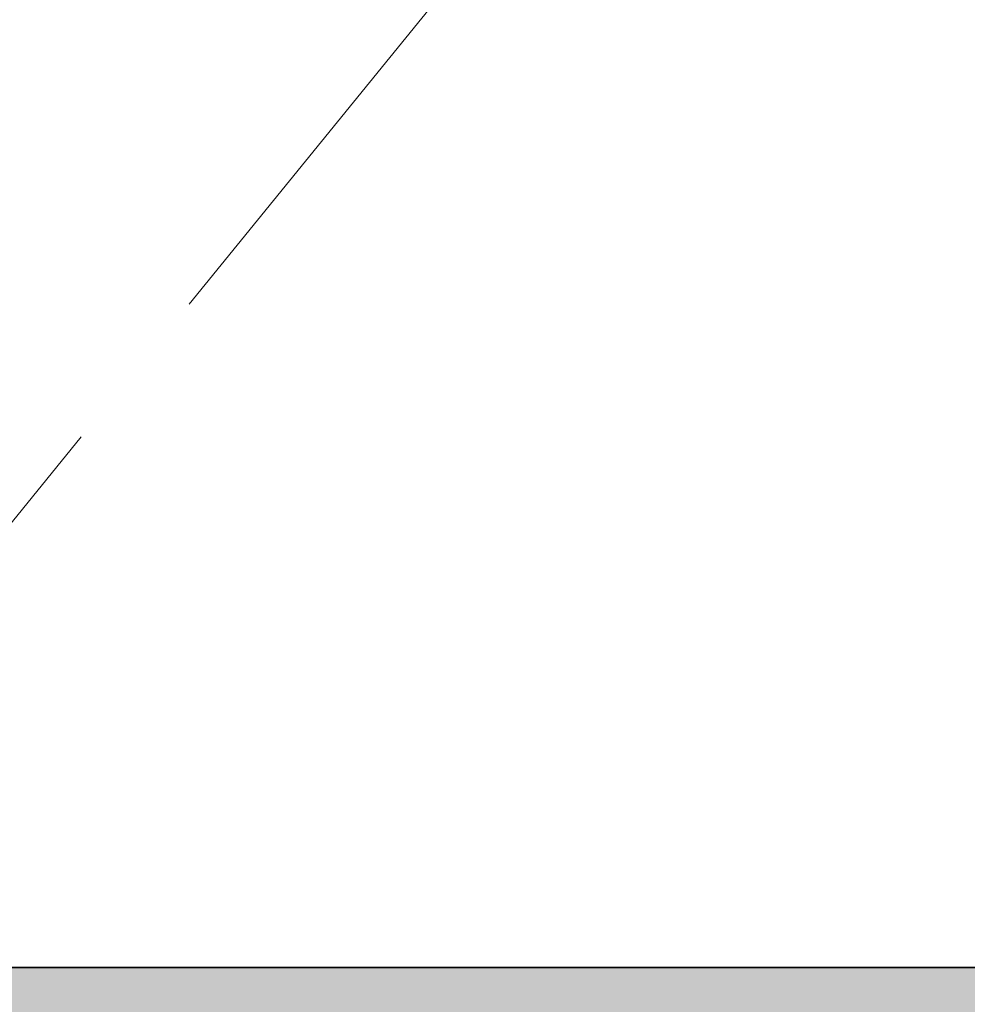
# Model space of a CAD drawing. Units: inches. Extents: x 2083 to 3317, y 1141 to 2115.
# Tile 77 of 256: x 2242.45 to 2259.08, y 1477.12 to 1494.39. Entities that reach past the tile are written whole.
import ezdxf

# ---------------------------------------------------------------- set-up
doc = ezdxf.new("R2010")
doc.units = ezdxf.units.IN
doc.linetypes.add('ACAD_ISO02W100', pattern=[15, 12, -3])
for name, color, linetype, lineweight in [('A-ANNO-DIMS', 2, 'Continuous', 18), ('A-FLOR-OPEN', 8, 'ACAD_ISO02W100', 13), ('A-WALL', 7, 'Continuous', 35)]:
    doc.layers.add(name, color=color, linetype=linetype, lineweight=lineweight)
doc.layers.add('A-WALL-PATT', color=251, linetype='Continuous', lineweight=13, true_color=0x636466)
doc.styles.get("Standard").update_dxf_attribs({"font": 'arial.ttf'})
doc.dimstyles.new('ISO-25', dxfattribs={"dimtxt": 12, "dimasz": 12, "dimexe": 1.25, "dimexo": 0.625, "dimtad": 1, "dimlunit": 3, "dimtxsty": 'Standard', "dimcen": 2.5, "dimadec": 0, "dimazin": 0, "dimtfac": 1, "dimtmove": 0, "dimatfit": 3, "dimfxl": 1, "dimarcsym": 0})

# ---------------------------------------------------------------- blocks, each defined once
blk = doc.blocks.new('*D30')
at = {"layer": 'A-ANNO-DIMS', "color": 0, "lineweight": -2, "transparency": 16777216}
for p, q in [((2240.018, 1445.274), (2240.018, 1448.046)), ((2254.329, 1445.274), (2254.329, 1448.046)), ((2228.018, 1446.796), (2216.018, 1446.796)), ((2240.018, 1446.796), (2254.329, 1446.796)), ((2266.329, 1446.796), (2413.765, 1446.796))]:
    blk.add_line(p, q, dxfattribs=at)
at = {"layer": 'A-ANNO-DIMS', "color": 0, "transparency": 16777216}
for points in [[(2228.018, 1448.796), (2228.018, 1444.796), (2240.018, 1446.796)], [(2266.329, 1448.796), (2266.329, 1444.796), (2254.329, 1446.796)]]:
    blk.add_solid(points, dxfattribs=at)
at = {"layer": 'Defpoints', "color": 0, "transparency": 16777216}
for p in [(2254.329, 1446.796), (2240.018, 1444.649), (2254.329, 1444.649)]:
    blk.add_point(p, dxfattribs=at)
at = {"layer": 'A-ANNO-DIMS', "color": 0, "transparency": 16777216, "insert": (2346.047, 1453.625), "char_height": 12, "attachment_point": 5}
blk.add_mtext('WC 1\'-2 1/2" TYP.', dxfattribs=at)
blk = doc.blocks.new('*D31')
at = {"layer": 'A-ANNO-DIMS', "color": 0, "lineweight": -2, "transparency": 16777216}
for p, q in [((2237.871, 1456.649), (2237.871, 1541.915)), ((2239.393, 1444.649), (2236.621, 1444.649)), ((2237.871, 1431.548), (2237.871, 1444.649)), ((2239.393, 1431.548), (2236.621, 1431.548)), ((2237.871, 1419.548), (2237.871, 1407.548))]:
    blk.add_line(p, q, dxfattribs=at)
at = {"layer": 'A-ANNO-DIMS', "color": 0, "transparency": 16777216}
for points in [[(2235.871, 1456.649), (2239.871, 1456.649), (2237.871, 1444.649)], [(2235.871, 1419.548), (2239.871, 1419.548), (2237.871, 1431.548)]]:
    blk.add_solid(points, dxfattribs=at)
at = {"layer": 'Defpoints', "color": 0, "transparency": 16777216}
for p in [(2237.871, 1444.649), (2240.018, 1444.649), (2240.018, 1431.548)]:
    blk.add_point(p, dxfattribs=at)
at = {"layer": 'A-ANNO-DIMS', "color": 0, "transparency": 16777216, "insert": (2231.217, 1505.282), "char_height": 12, "attachment_point": 5, "rotation": 90}
blk.add_mtext('1\'-1" TYP.', dxfattribs=at)
blk = doc.blocks.new('*D45')
at = {"layer": 'A-ANNO-DIMS', "color": 0, "lineweight": -2, "transparency": 16777216}
for p, q in [((2235.96, 1478.386), (2235.96, 1531.361)), ((2418.96, 1478.386), (2418.96, 1531.361)), ((2247.96, 1530.111), (2406.96, 1530.111))]:
    blk.add_line(p, q, dxfattribs=at)
at = {"layer": 'A-ANNO-DIMS', "color": 0, "transparency": 16777216}
for points in [[(2247.96, 1532.111), (2247.96, 1528.111), (2235.96, 1530.111)], [(2406.96, 1532.111), (2406.96, 1528.111), (2418.96, 1530.111)]]:
    blk.add_solid(points, dxfattribs=at)
at = {"layer": 'Defpoints', "color": 0, "transparency": 16777216}
for p in [(2418.96, 1530.111), (2235.96, 1477.761), (2418.96, 1477.761)]:
    blk.add_point(p, dxfattribs=at)
at = {"layer": 'A-ANNO-DIMS', "color": 0, "transparency": 16777216, "insert": (2327.46, 1536.867), "char_height": 12, "attachment_point": 5}
blk.add_mtext('15\'-3"', dxfattribs=at)
blk = doc.blocks.new('*D62')
at = {"layer": 'A-ANNO-DIMS', "color": 0, "lineweight": -2, "transparency": 16777216}
for p, q in [((2235.96, 1469.386), (2235.96, 1522.361)), ((2379.96, 1469.386), (2379.96, 1522.361)), ((2247.96, 1521.111), (2367.96, 1521.111))]:
    blk.add_line(p, q, dxfattribs=at)
at = {"layer": 'A-ANNO-DIMS', "color": 0, "transparency": 16777216}
for points in [[(2247.96, 1523.111), (2247.96, 1519.111), (2235.96, 1521.111)], [(2367.96, 1523.111), (2367.96, 1519.111), (2379.96, 1521.111)]]:
    blk.add_solid(points, dxfattribs=at)
at = {"layer": 'Defpoints', "color": 0, "transparency": 16777216}
for p in [(2379.96, 1521.111), (2235.96, 1468.761), (2379.96, 1468.761)]:
    blk.add_point(p, dxfattribs=at)
at = {"layer": 'A-ANNO-DIMS', "color": 0, "transparency": 16777216, "insert": (2307.96, 1527.863), "char_height": 12, "attachment_point": 5}
blk.add_mtext('12\'-0"', dxfattribs=at)
blk = doc.blocks.new('*D64')
at = {"layer": 'A-ANNO-DIMS', "color": 0, "lineweight": -2, "transparency": 16777216}
for p, q in [((2236.585, 1702.761), (2289.56, 1702.761)), ((2288.31, 1690.761), (2288.31, 1489.761)), ((2236.585, 1477.761), (2289.56, 1477.761))]:
    blk.add_line(p, q, dxfattribs=at)
at = {"layer": 'A-ANNO-DIMS', "color": 0, "transparency": 16777216}
for points in [[(2286.31, 1690.761), (2290.31, 1690.761), (2288.31, 1702.761)], [(2286.31, 1489.761), (2290.31, 1489.761), (2288.31, 1477.761)]]:
    blk.add_solid(points, dxfattribs=at)
at = {"layer": 'Defpoints', "color": 0, "transparency": 16777216}
for p in [(2235.96, 1702.761), (2235.96, 1477.761), (2288.31, 1477.761)]:
    blk.add_point(p, dxfattribs=at)
at = {"layer": 'A-ANNO-DIMS', "color": 0, "transparency": 16777216, "insert": (2281.558, 1590.261), "char_height": 12, "attachment_point": 5, "rotation": 90}
blk.add_mtext('18\'-9"', dxfattribs=at)

msp = doc.modelspace()

# ---------------------------------------------------------------- hatches: boundary and pattern name
at = {"layer": 'A-WALL-PATT'}
h = msp.add_hatch(color=256, dxfattribs=at)
h.dxf.hatch_style = 1
h.paths.add_polyline_path([(3126.96, 2020.761), (2748.96, 2020.761), (2604.96, 2020.761), (2226.96, 2020.761), (2226.96, 1702.761), (2466.96, 1702.761), (2466.96, 1582.761), (2418.96, 1582.761), (2418.96, 1477.761), (2226.96, 1477.761), (2226.96, 1263.261), (2544.96, 1263.261), (2544.96, 1411.761), (2604.96, 1411.761), (2685.96, 1411.761), (2685.96, 1420.761), (2604.96, 1420.761), (2604.96, 1573.761), (2604.96, 1702.761), (2604.96, 2011.761), (2748.96, 2011.761), (2748.96, 1702.761), (2862.96, 1702.761), (2862.96, 1621.761), (2871.96, 1621.761), (2871.96, 1702.761), (2883.96, 1702.761), (2883.96, 1706.939, -0.026459), (2883.96, 1711.761), (2757.96, 1711.761), (2757.96, 1807.761), (2787.96, 1807.761), (2787.96, 1812.261), (2757.96, 1812.261), (2757.96, 2011.761), (2877.96, 2011.761), (2877.96, 1812.261), (2847.96, 1812.261), (2847.96, 1807.761), (2889.836, 1807.761), (2889.836, 1812.261), (2882.46, 1812.261), (2882.46, 2011.761), (3117.96, 2011.761), (3117.96, 1812.261), (2937.836, 1812.261), (2937.836, 1807.761), (2995.71, 1807.761), (2995.71, 1796.118), (3000.21, 1796.118), (3000.21, 1807.761), (3117.96, 1807.761), (3117.96, 1711.761), (3000.21, 1711.761), (3000.21, 1760.118), (2998.573, 1760.118, -0.020711), (2995.71, 1760.118), (2995.71, 1711.761), (2931.96, 1711.761), (2931.96, 1702.761), (3126.96, 1702.761)])
h.paths.add_polyline_path([(2471.46, 2011.761), (2471.46, 1810.011), (2462.717, 1810.011), (2462.717, 1805.511), (2505.96, 1805.511), (2505.96, 1810.011), (2475.96, 1810.011), (2475.96, 2011.761), (2595.96, 2011.761), (2595.96, 1810.011), (2565.96, 1810.011), (2565.96, 1805.511), (2595.96, 1805.511), (2595.96, 1711.761), (2235.96, 1711.761), (2235.96, 1805.511), (2353.71, 1805.511), (2353.71, 1796.054), (2358.21, 1796.054), (2358.21, 1805.511), (2414.717, 1805.511), (2414.717, 1810.011), (2235.96, 1810.011), (2235.96, 2011.761)], flags=16)
h.paths.add_polyline_path([(2270.205, 1994.61), (2270.205, 1970.61), (2246.205, 1970.61), (2246.205, 1994.61)], flags=0)
edge = h.paths.add_edge_path(flags=0)
edge.add_ellipse((2332.027, 1899.798), major_axis=(-3.043, 3.043), ratio=0.168252, start_angle=-161.3322, end_angle=-156.3071, ccw=False)
edge.add_ellipse((2333.082, 1898.744), major_axis=(-1.055, 1.055), ratio=0.453532, start_angle=-123.371, end_angle=-94.1591)
edge = h.paths.add_edge_path(flags=0)
edge.add_ellipse((2332.027, 1968.876), major_axis=(3.043, 3.043), ratio=0.168252, start_angle=18.6678, end_angle=23.6929)
edge.add_spline(control_points=[(2332.926, 1970.691), (2332.227, 1970.336), (2330.894, 1969.659), (2328.413, 1970.932), (2327.204, 1967.749), (2324.71, 1969.956), (2322.533, 1967.012), (2320.013, 1971.296), (2317.68, 1968.158), (2316.041, 1967.102), (2315.427, 1966.81)], knot_values=[0, 0, 0, 0, 2.267059, 4.324559, 6.685584, 8.878641, 11.121502, 14.300359, 17.755284, 19.732645, 19.732645, 19.732645, 19.732645], degree=3, periodic=0)
edge.add_ellipse((2332.027, 1968.876), major_axis=(3.043, 3.043), ratio=0.168252, start_angle=18.6678, end_angle=23.6929, ccw=False)
edge.add_ellipse((2333.082, 1969.931), major_axis=(1.055, 1.055), ratio=0.453532, start_angle=56.629, end_angle=85.8409, ccw=False)
edge = h.paths.add_edge_path(flags=0)
edge.add_spline(control_points=[(2296.428, 1967.988), (2293.628, 1965.336), (2287.704, 1959.727), (2299.744, 1949.996), (2294.533, 1935.669), (2290.573, 1920.604), (2293.394, 1909.974), (2296.185, 1904.967)], knot_values=[0.099185, 0.099185, 0.099185, 0.099185, 0.345301, 0.619822, 0.982653, 1.386093, 1.810555, 1.810555, 1.810555, 1.810555], degree=3, periodic=0)
edge.add_spline(control_points=[(2296.185, 1904.967), (2297.384, 1902.619), (2298.001, 1901.949), (2298.553, 1901.468)], knot_values=[0.006246, 0.006246, 0.006246, 0.006246, 0.055476, 0.055476, 0.055476, 0.055476], degree=3, periodic=0)
edge.add_spline(control_points=[(2298.553, 1901.468), (2297.259, 1900.923), (2295.225, 1900.232), (2293.06, 1900.614), (2292.101, 1900.788), (2292.09, 1900.791)], knot_values=[0.312835, 0.312835, 0.312835, 0.312835, 0.40178, 0.474987, 0.475903, 0.475903, 0.475903, 0.475903], degree=3, periodic=0)
edge.add_arc((2292.794, 1904.664), 3.937, 215.4209, 259.6982, ccw=False)
edge.add_spline(control_points=[(2289.585, 1902.382), (2289.477, 1902.535), (2289.368, 1902.688), (2289.261, 1902.841)], knot_values=[0.102872, 0.102872, 0.102872, 0.102872, 0.116896, 0.116896, 0.116896, 0.116896], degree=3, periodic=0)
edge.add_spline(control_points=[(2289.261, 1902.841), (2288.687, 1902.55), (2287.64, 1902.02), (2285.881, 1901.874), (2283.853, 1901.504), (2281.72, 1899.711), (2278.467, 1899.493), (2276.157, 1901.883), (2272.259, 1899.804), (2267.778, 1901.843), (2262.244, 1900.184), (2257.415, 1901.782), (2254.318, 1900.726), (2253.178, 1900.337)], knot_values=[0, 0, 0, 0, 1.907977, 3.477176, 5.261074, 7.972851, 11.680248, 13.717921, 16.939592, 22.789562, 27.502503, 33.595215, 37.145618, 37.145618, 37.145618, 37.145618], degree=3, periodic=0)
edge.add_line((2253.178, 1900.337), (2250.244, 1902.841))
edge.add_line((2250.244, 1902.841), (2250.244, 1965.833))
edge.add_line((2250.244, 1965.833), (2253.178, 1968.337))
edge.add_spline(control_points=[(2253.178, 1968.337), (2254.318, 1967.948), (2257.415, 1966.892), (2262.244, 1968.49), (2267.778, 1966.831), (2271.527, 1968.537), (2273.876, 1967.828), (2274.207, 1967.728)], knot_values=[0, 0, 0, 0, 0.09018, 0.244935, 0.364644, 0.513233, 0.537855, 0.537855, 0.537855, 0.537855], degree=3, periodic=0)
edge.add_arc((2274.353, 1963.793), 3.937, 72.0511, 92.1279, ccw=False)
edge.add_arc((2281.297, 1985.23), 18.596, 252.0511, 288.5657)
edge.add_arc((2292.317, 1956.029), 12.646, 71.0268, 113.7782, ccw=False)
edge = h.paths.add_edge_path(flags=0)
edge.add_spline(control_points=[(2274.899, 1951.856), (2275.066, 1951.617), (2275.233, 1951.377), (2275.398, 1951.136)], knot_values=[1.409916, 1.409916, 1.409916, 1.409916, 1.43159, 1.43159, 1.43159, 1.43159], degree=3, periodic=0)
edge.add_spline(control_points=[(2275.398, 1951.136), (2275.792, 1950.562), (2276.179, 1949.984), (2276.546, 1949.397)], knot_values=[1.358238, 1.358238, 1.358238, 1.358238, 1.409916, 1.409916, 1.409916, 1.409916], degree=3, periodic=0)
edge.add_line((2276.546, 1949.397), (2277.437, 1947.862))
edge.add_spline(control_points=[(2277.437, 1947.862), (2276.304, 1945.673), (2274.64, 1942.427), (2274.632, 1938.094), (2272.799, 1930.852), (2274.356, 1943.897), (2275.948, 1947.923), (2276.546, 1949.397)], knot_values=[0.005632, 0.005632, 0.005632, 0.005632, 0.186014, 0.266002, 0.357087, 0.59639, 0.739732, 0.739732, 0.739732, 0.739732], degree=3, periodic=0)
edge.add_spline(control_points=[(2276.546, 1949.397), (2276.179, 1949.984), (2275.792, 1950.562), (2275.398, 1951.136)], knot_values=[1.358238, 1.358238, 1.358238, 1.358238, 1.409916, 1.409916, 1.409916, 1.409916], degree=3, periodic=0)
edge.add_spline(control_points=[(2275.398, 1951.136), (2274.943, 1950.08), (2274.208, 1948.025), (2273.935, 1944.851), (2272.469, 1937.627), (2273.466, 1945.696), (2274.701, 1951.059), (2274.899, 1951.856)], knot_values=[0.104364, 0.104364, 0.104364, 0.104364, 0.189636, 0.269624, 0.36071, 0.600013, 0.644622, 0.644622, 0.644622, 0.644622], degree=3, periodic=0)
h.paths.add_polyline_path([(2269.168, 1963.128, -0.357527), (2268.171, 1960.976, -0.092561), (2268.171, 1939.436, -0.357527), (2269.168, 1937.285, -0.357527), (2267.016, 1938.282, -0.164785), (2254.686, 1938.282, -0.357527), (2252.534, 1937.285, -0.357527), (2253.531, 1939.436, -0.092561), (2253.531, 1960.976, -0.357527), (2252.534, 1963.128, -0.357527), (2254.686, 1962.131, -0.164785), (2267.016, 1962.131, -0.357527)], flags=0)
h.paths.add_polyline_path([(2248.874, 1967.802), (2248.874, 1957.028), (2249.458, 1957.028), (2249.458, 1911.647), (2248.874, 1911.647), (2248.874, 1900.873), (2246.512, 1900.873, 0.197327), (2244.15, 1902.457), (2244.15, 1966.218, 0.197327), (2246.512, 1967.802)], flags=0)
h.paths.add_polyline_path([(2269.168, 1931.389, -0.357527), (2268.171, 1929.238, -0.092561), (2268.171, 1907.698, -0.357527), (2269.168, 1905.547, -0.357527), (2267.016, 1906.544, -0.164785), (2254.686, 1906.544, -0.357527), (2252.534, 1905.547, -0.357527), (2253.531, 1907.698, -0.092561), (2253.531, 1929.238, -0.357527), (2252.534, 1931.389, -0.357527), (2254.686, 1930.392, -0.164785), (2267.016, 1930.392, -0.357527)], flags=0)
edge = h.paths.add_edge_path(flags=0)
edge.add_spline(control_points=[(2276.197, 1906.724), (2276.168, 1909.029), (2276.114, 1913.372), (2270.598, 1924.925), (2273.905, 1919.013), (2275.922, 1916.262), (2275.475, 1912.402), (2277.258, 1910.381), (2276.696, 1908.225), (2276.646, 1906.813), (2276.618, 1906.008)], knot_values=[0, 0, 0, 0, 8.61026, 16.221274, 18.843057, 23.804898, 27.440828, 29.356102, 31.203478, 33.650687, 33.650687, 33.650687, 33.650687], degree=3, periodic=0)
edge.add_spline(control_points=[(2276.618, 1906.008), (2276.623, 1905.624), (2276.498, 1904.629), (2275.442, 1903.855), (2274.937, 1903.08), (2274.859, 1902.841)], knot_values=[0.156488, 0.156488, 0.156488, 0.156488, 0.184398, 0.231376, 0.250598, 0.250598, 0.250598, 0.250598], degree=3, periodic=0)
edge.add_line((2274.859, 1902.841), (2276.506, 1902.841))
edge.add_spline(control_points=[(2276.506, 1902.841), (2276.788, 1903.085), (2277.665, 1904.125), (2278.25, 1904.341), (2277.654, 1908.527), (2278.156, 1906.228), (2278.1, 1905.286), (2278.847, 1904.069), (2277.857, 1903.415), (2277.874, 1902.991), (2277.904, 1902.841)], knot_values=[0.059574, 0.059574, 0.059574, 0.059574, 0.080753, 0.103741, 0.16972, 0.176036, 0.207137, 0.240474, 0.262341, 0.27366, 0.27366, 0.27366, 0.27366], degree=3, periodic=0)
edge.add_line((2277.904, 1902.841), (2280.03, 1902.841))
edge.add_spline(control_points=[(2280.03, 1902.841), (2279.888, 1903.088), (2279.499, 1903.982), (2280.152, 1905.939), (2278.104, 1909.658), (2279.762, 1907.185), (2280.328, 1904.875), (2280.485, 1903.49), (2281.463, 1903.249), (2281.758, 1902.936), (2281.834, 1902.841)], knot_values=[0.013856, 0.013856, 0.013856, 0.013856, 0.034874, 0.088867, 0.107879, 0.126738, 0.158714, 0.193757, 0.217487, 0.226722, 0.226722, 0.226722, 0.226722], degree=3, periodic=0)
edge.add_spline(control_points=[(2281.834, 1902.841), (2281.788, 1902.827), (2281.647, 1902.783), (2281.396, 1902.859), (2281.088, 1902.985), (2280.721, 1903.061), (2280.333, 1903.026), (2280.125, 1902.899), (2280.03, 1902.841)], knot_values=[0, 0, 0, 0, 0.14413, 0.435517, 0.749276, 1.153046, 1.548371, 1.878348, 1.878348, 1.878348, 1.878348], degree=3, periodic=0)
edge.add_line((2280.03, 1902.841), (2277.904, 1902.841))
edge.add_spline(control_points=[(2277.904, 1902.841), (2277.893, 1902.796), (2277.865, 1902.68), (2277.607, 1902.687), (2277.274, 1902.801), (2276.838, 1902.62), (2276.584, 1902.789), (2276.506, 1902.841)], knot_values=[0, 0, 0, 0, 0.127189, 0.326199, 0.628009, 1.24357, 1.515331, 1.515331, 1.515331, 1.515331], degree=3, periodic=0)
edge.add_line((2276.506, 1902.841), (2274.859, 1902.841))
edge.add_spline(control_points=[(2274.859, 1902.841), (2274.814, 1902.899), (2274.725, 1903.013), (2274.493, 1903.119), (2274.244, 1902.961), (2273.937, 1903.185), (2273.614, 1902.983), (2273.408, 1902.883), (2273.322, 1902.841)], knot_values=[0, 0, 0, 0, 0.21843, 0.436957, 0.687977, 0.990379, 1.398396, 1.69185, 1.69185, 1.69185, 1.69185], degree=3, periodic=0)
edge.add_spline(control_points=[(2273.322, 1902.841), (2273.617, 1903.446), (2274.274, 1904.538), (2276.027, 1904.574), (2276.207, 1906.584), (2276.197, 1906.724)], knot_values=[0.012227, 0.012227, 0.012227, 0.012227, 0.059472, 0.106218, 0.134458, 0.134458, 0.134458, 0.134458], degree=3, periodic=0)
h.paths.add_polyline_path([(2270.776, 1897.79), (2270.776, 1873.79), (2246.776, 1873.79), (2246.776, 1897.79)], flags=0)
h.paths.add_polyline_path([(2353.71, 1760.005), (2353.71, 1760.054), (2358.21, 1760.054, -0.033729)], flags=0)
h.paths.add_polyline_path([(2321.819, 1737.529), (2341.995, 1737.529, -0.414214), (2343.203, 1736.321), (2343.203, 1721.021, -0.414214), (2341.995, 1719.813), (2321.819, 1719.813, -0.414214), (2320.611, 1721.021), (2320.611, 1736.321, -0.414214)], flags=0)
h.paths.add_polyline_path([(2324.235, 1736.321), (2339.579, 1736.321, -0.414214), (2341.995, 1733.905), (2341.995, 1725.45, -0.414214), (2339.579, 1723.034), (2333.681, 1723.034), (2333.845, 1722.045, -0.870646), (2335.425, 1721.826, -0.767327), (2333.923, 1721.423), (2331.291, 1721.423, -0.767327), (2329.788, 1721.826, -0.870646), (2331.368, 1722.045), (2331.533, 1723.034), (2324.235, 1723.034, -0.414214), (2321.819, 1725.45), (2321.819, 1733.905, -0.414214)], flags=0)
h.paths.add_polyline_path([(2570.484, 1928.615), (2589.684, 1928.615), (2590.169, 1928.615), (2590.169, 1904.993), (2570.484, 1904.993)], flags=0)
h.paths.add_polyline_path([(2574.447, 1927.264, -1), (2572.829, 1927.264, -1)], flags=0)
h.paths.add_polyline_path([(2573.09, 1926.941), (2573.925, 1927.776), (2574.148, 1927.553), (2573.313, 1926.718)], flags=0)
h.paths.add_polyline_path([(2578.779, 1919.73, -1), (2571.592, 1919.73, -1)], flags=0)
h.paths.add_polyline_path([(2578.385, 1919.73, -1), (2571.985, 1919.73, -1)], flags=0)
h.paths.add_polyline_path([(2331.596, 1729.476, -1), (2333.618, 1729.476, -1)], flags=0)
h.paths.add_polyline_path([(2578.034, 1927.264, -1), (2576.416, 1927.264, -1)], flags=0)
h.paths.add_polyline_path([(2576.689, 1927.531), (2576.912, 1927.754), (2577.747, 1926.919), (2577.524, 1926.696)], flags=0)
h.paths.add_polyline_path([(2578.139, 1909.86, -1), (2572.232, 1909.86, -1)], flags=0)
h.paths.add_polyline_path([(2577.745, 1909.86, -1), (2572.625, 1909.86, -1)], flags=0)
h.paths.add_polyline_path([(2583.798, 1927.264, -1), (2582.179, 1927.264, -1)], flags=0)
h.paths.add_polyline_path([(2582.719, 1927.754), (2583.554, 1926.919), (2583.331, 1926.696), (2582.496, 1927.531)], flags=0)
h.paths.add_polyline_path([(2582.496, 1927.531), (2582.719, 1927.754), (2583.554, 1926.919), (2583.331, 1926.696)], flags=0)
h.paths.add_polyline_path([(2587.739, 1920.53, -1), (2581.832, 1920.53, -1)], flags=0)
h.paths.add_polyline_path([(2587.345, 1920.53, -1), (2582.225, 1920.53, -1)], flags=0)
h.paths.add_polyline_path([(2587.385, 1927.264, -1), (2585.766, 1927.264, -1)], flags=0)
h.paths.add_polyline_path([(2586.082, 1926.98), (2586.917, 1927.815), (2587.14, 1927.593), (2586.305, 1926.758)], flags=0)
h.paths.add_polyline_path([(2588.379, 1910.66, -1), (2581.192, 1910.66, -1)], flags=0)
h.paths.add_polyline_path([(2587.985, 1910.66, -1), (2581.585, 1910.66, -1)], flags=0)
h.paths.add_polyline_path([(2417.168, 1729.478), (2437.344, 1729.478, -0.414214), (2438.552, 1728.27), (2438.552, 1712.969, -0.414214), (2437.344, 1711.761), (2417.168, 1711.761, -0.414214), (2415.96, 1712.969), (2415.96, 1728.27, -0.414214)], flags=0)
h.paths.add_polyline_path([(2419.584, 1728.27), (2434.928, 1728.27, -0.414214), (2437.344, 1725.854), (2437.344, 1717.398, -0.414214), (2434.928, 1714.983), (2429.029, 1714.983), (2429.194, 1713.994, -0.870646), (2430.774, 1713.775, -0.767327), (2429.271, 1713.372), (2426.64, 1713.372, -0.767327), (2425.137, 1713.775, -0.870646), (2426.717, 1713.994), (2426.882, 1714.983), (2419.584, 1714.983, -0.414214), (2417.168, 1717.398), (2417.168, 1725.854, -0.414214)], flags=0)
h.paths.add_polyline_path([(2419.584, 1728.27), (2434.928, 1728.27, -0.414214), (2437.344, 1725.854), (2437.344, 1717.398, -0.414214), (2434.928, 1714.983), (2429.029, 1714.983), (2428.358, 1719.009), (2427.553, 1719.009), (2426.882, 1714.983), (2419.584, 1714.983, -0.414214), (2417.168, 1717.398), (2417.168, 1725.854, -0.414214)], flags=0)
h.paths.add_polyline_path([(2426.944, 1721.425, -1), (2428.967, 1721.425, -1)], flags=0)
h.paths.add_polyline_path([(2475.96, 1702.761), (2595.96, 1702.761), (2595.96, 1582.761), (2475.96, 1582.761)], flags=16)
h.paths.add_polyline_path([(2427.96, 1573.761), (2595.96, 1573.761), (2595.96, 1468.761), (2595.96, 1420.761), (2384.46, 1420.761), (2384.46, 1468.761), (2427.96, 1468.761)], flags=16)
h.paths.add_polyline_path([(2379.96, 1468.761), (2379.96, 1420.761), (2235.96, 1420.761), (2235.96, 1468.761)], flags=16)
h.paths.add_polyline_path([(2317.816, 1466.696), (2337.992, 1466.696, -0.414214), (2339.2, 1465.488), (2339.2, 1450.187, -0.414214), (2337.992, 1448.979), (2317.816, 1448.979, -0.414214), (2316.608, 1450.187), (2316.608, 1465.488, -0.414214)], flags=0)
h.paths.add_polyline_path([(2320.232, 1465.488), (2335.576, 1465.488, -0.414214), (2337.992, 1463.072), (2337.992, 1454.616, -0.414214), (2335.576, 1452.2), (2329.677, 1452.2), (2329.842, 1451.212, -0.870646), (2331.422, 1450.992, -0.767327), (2329.92, 1450.59), (2327.288, 1450.59, -0.767327), (2325.785, 1450.992, -0.870646), (2327.365, 1451.212), (2327.53, 1452.2), (2320.232, 1452.2, -0.414214), (2317.816, 1454.616), (2317.816, 1463.072, -0.414214)], flags=0)
h.paths.add_polyline_path([(2320.232, 1465.488), (2335.576, 1465.488, -0.414214), (2337.992, 1463.072), (2337.992, 1454.616, -0.414214), (2335.576, 1452.2), (2329.677, 1452.2), (2329.006, 1456.227), (2328.201, 1456.227), (2327.53, 1452.2), (2320.232, 1452.2, -0.414214), (2317.816, 1454.616), (2317.816, 1463.072, -0.414214)], flags=0)
h.paths.add_polyline_path([(2327.593, 1458.643, -1), (2329.615, 1458.643, -1)], flags=0)
h.paths.add_polyline_path([(2244.412, 1433.34), (2241.921, 1433.34, -0.414214), (2240.018, 1435.244), (2240.018, 1440.953, -0.414211), (2241.921, 1442.856), (2244.412, 1442.856, -1.976472)], flags=0)
h.paths.add_polyline_path([(2245.357, 1434.398, -0.414214), (2245.357, 1441.799, -2.144098)], flags=0)
h.paths.add_polyline_path([(2535.96, 1416.261), (2535.96, 1272.261), (2235.96, 1272.261), (2235.96, 1416.261)], flags=16)
h.paths.add_polyline_path([(2260.12, 1384.293), (2260.12, 1362.039), (2237.865, 1362.039), (2237.865, 1384.293)], flags=0)
edge = h.paths.add_edge_path(flags=0)
edge.add_line((2318.252, 1362.093), (2318.146, 1362.001))
edge.add_ellipse((2317.445, 1360.431), major_axis=(2.822, 2.822), ratio=0.168252, start_angle=18.6678, end_angle=20.9481, ccw=False)
edge.add_ellipse((2318.423, 1361.409), major_axis=(0.978, 0.978), ratio=0.453532, start_angle=56.629, end_angle=70.2262, ccw=False)
edge = h.paths.add_edge_path(flags=0)
edge.add_line((2319.107, 1295.571), (2319.015, 1295.677))
edge.add_ellipse((2317.445, 1296.378), major_axis=(-2.822, 2.822), ratio=0.168252, start_angle=-161.3322, end_angle=-159.0519, ccw=False)
edge.add_ellipse((2318.423, 1295.4), major_axis=(-0.978, 0.978), ratio=0.453532, start_angle=-123.371, end_angle=-109.7738)
edge = h.paths.add_edge_path(flags=0)
edge.add_spline(control_points=[(2284.21, 1301.17), (2284.581, 1300.445), (2284.891, 1299.892), (2285.16, 1299.461)], knot_values=[0.039066, 0.039066, 0.039066, 0.039066, 0.055476, 0.055476, 0.055476, 0.055476], degree=3, periodic=0)
edge.add_line((2285.16, 1299.461), (2284.21, 1301.17))
edge = h.paths.add_edge_path(flags=0)
edge.add_line((2280.412, 1297.298), (2283.37, 1297.036))
edge.add_line((2283.37, 1297.036), (2286.406, 1297.926))
edge.add_spline(control_points=[(2286.406, 1297.926), (2285.305, 1297.463), (2284.345, 1297.129), (2283.37, 1297.036)], knot_values=[0.394369, 0.394369, 0.394369, 0.394369, 0.475903, 0.475903, 0.475903, 0.475903], degree=3, periodic=0)
edge.add_spline(control_points=[(2283.37, 1297.036), (2283.281, 1297.028), (2282.316, 1296.957), (2281.313, 1297.134), (2280.423, 1297.296), (2280.412, 1297.298)], knot_values=[0.312835, 0.312835, 0.312835, 0.312835, 0.320246, 0.393453, 0.394369, 0.394369, 0.394369, 0.394369], degree=3, periodic=0)
edge = h.paths.add_edge_path(flags=0)
edge.add_line((2284.436, 1359.607), (2280.446, 1355.328))
edge.add_line((2280.446, 1355.328), (2279.58, 1351.018))
edge.add_line((2279.58, 1351.018), (2282.413, 1346.58))
edge.add_spline(control_points=[(2282.413, 1346.58), (2283.153, 1345.589), (2284.253, 1344.029), (2284.801, 1342.387), (2284.935, 1341.806)], knot_values=[1.240098, 1.240098, 1.240098, 1.240098, 1.332892, 1.382712, 1.382712, 1.382712, 1.382712], degree=3, periodic=0)
edge.add_spline(control_points=[(2284.935, 1341.806), (2285.319, 1340.141), (2285.233, 1338.409), (2284.91, 1336.654)], knot_values=[1.097484, 1.097484, 1.097484, 1.097484, 1.240098, 1.240098, 1.240098, 1.240098], degree=3, periodic=0)
edge.add_spline(control_points=[(2284.91, 1336.654), (2284.587, 1334.899), (2284.027, 1333.12), (2283.463, 1331.361)], knot_values=[0.95487, 0.95487, 0.95487, 0.95487, 1.097484, 1.097484, 1.097484, 1.097484], degree=3, periodic=0)
edge.add_line((2283.463, 1331.361), (2281.89, 1326.153))
edge.add_line((2281.89, 1326.153), (2280.756, 1321.056))
edge.add_line((2280.756, 1321.056), (2280.299, 1316.002))
edge.add_line((2280.299, 1316.002), (2280.716, 1310.95))
edge.add_line((2280.716, 1310.95), (2282.028, 1305.972))
edge.add_line((2282.028, 1305.972), (2284.21, 1301.17))
edge.add_spline(control_points=[(2284.21, 1301.17), (2283.341, 1302.73), (2282.612, 1304.336), (2282.028, 1305.972)], knot_values=[0.099185, 0.099185, 0.099185, 0.099185, 0.241799, 0.241799, 0.241799, 0.241799], degree=3, periodic=0)
edge.add_spline(control_points=[(2282.028, 1305.972), (2281.444, 1307.608), (2281.005, 1309.273), (2280.716, 1310.95)], knot_values=[0.241799, 0.241799, 0.241799, 0.241799, 0.384413, 0.384413, 0.384413, 0.384413], degree=3, periodic=0)
edge.add_spline(control_points=[(2280.716, 1310.95), (2280.433, 1312.588), (2280.289, 1314.277), (2280.299, 1315.962), (2280.299, 1316.002)], knot_values=[0.384413, 0.384413, 0.384413, 0.384413, 0.523647, 0.527028, 0.527028, 0.527028, 0.527028], degree=3, periodic=0)
edge.add_spline(control_points=[(2280.299, 1316.002), (2280.312, 1317.687), (2280.478, 1319.368), (2280.756, 1321.056)], knot_values=[0.527028, 0.527028, 0.527028, 0.527028, 0.669642, 0.669642, 0.669642, 0.669642], degree=3, periodic=0)
edge.add_spline(control_points=[(2280.756, 1321.056), (2281.035, 1322.744), (2281.426, 1324.44), (2281.89, 1326.153)], knot_values=[0.669642, 0.669642, 0.669642, 0.669642, 0.812256, 0.812256, 0.812256, 0.812256], degree=3, periodic=0)
edge.add_spline(control_points=[(2281.89, 1326.153), (2282.264, 1327.533), (2282.788, 1329.262), (2283.353, 1331.018), (2283.463, 1331.361)], knot_values=[0.812256, 0.812256, 0.812256, 0.812256, 0.927087, 0.95487, 0.95487, 0.95487, 0.95487], degree=3, periodic=0)
edge.add_line((2283.463, 1331.361), (2284.91, 1336.654))
edge.add_line((2284.91, 1336.654), (2284.935, 1341.806))
edge.add_line((2284.935, 1341.806), (2282.413, 1346.58))
edge.add_spline(control_points=[(2282.413, 1346.58), (2281.275, 1348.104), (2280.078, 1349.57), (2279.58, 1351.018)], knot_values=[1.382712, 1.382712, 1.382712, 1.382712, 1.525326, 1.525326, 1.525326, 1.525326], degree=3, periodic=0)
edge.add_spline(control_points=[(2279.58, 1351.018), (2279.443, 1351.415), (2279.136, 1352.857), (2279.735, 1354.29), (2280.446, 1355.328)], knot_values=[1.525326, 1.525326, 1.525326, 1.525326, 1.564439, 1.667941, 1.667941, 1.667941, 1.667941], degree=3, periodic=0)
edge.add_spline(control_points=[(2280.446, 1355.328), (2281.426, 1356.758), (2282.931, 1358.183), (2284.436, 1359.607)], knot_values=[1.667941, 1.667941, 1.667941, 1.667941, 1.810555, 1.810555, 1.810555, 1.810555], degree=3, periodic=0)
edge.add_arc((2280.623, 1348.518), 11.726, 71.0268, 113.7782)
edge.add_arc((2270.405, 1375.595), 17.244, 252.0511, 288.5657, ccw=False)
edge.add_arc((2263.966, 1355.718), 3.651, 72.0511, 92.1279)
edge.add_arc((2263.966, 1355.718), 3.651, 92.1279, 177.9851)
edge.add_spline(control_points=[(2260.318, 1355.846), (2260.26, 1354.221), (2260.551, 1350.187), (2262.999, 1346.766), (2264.473, 1344.649)], knot_values=[1.43159, 1.43159, 1.43159, 1.43159, 1.564144, 1.770695, 1.770695, 1.770695, 1.770695], degree=3, periodic=0)
edge.add_line((2264.473, 1344.649), (2264.936, 1343.983))
edge.add_spline(control_points=[(2263.801, 1340.248), (2263.843, 1340.514), (2264.067, 1341.756), (2264.513, 1343.002), (2264.935, 1343.981)], knot_values=[0.53657, 0.53657, 0.53657, 0.53657, 0.559349, 0.644622, 0.644622, 0.644622, 0.644622], degree=3, periodic=0)
edge.add_spline(control_points=[(2264.935, 1343.981), (2265.118, 1343.715), (2265.299, 1343.448), (2265.477, 1343.179)], knot_values=[1.384077, 1.384077, 1.384077, 1.384077, 1.409916, 1.409916, 1.409916, 1.409916], degree=3, periodic=0)
edge.add_spline(control_points=[(2265.477, 1343.179), (2265.655, 1342.911), (2265.829, 1342.641), (2265.999, 1342.369)], knot_values=[1.358238, 1.358238, 1.358238, 1.358238, 1.384077, 1.384077, 1.384077, 1.384077], degree=3, periodic=0)
edge.add_line((2265.999, 1342.369), (2266.826, 1340.946))
edge.add_spline(control_points=[(2266.826, 1340.946), (2268.894, 1337.09), (2271.398, 1325.843), (2270.516, 1310.569), (2275.919, 1301.861), (2277.79, 1299.199)], knot_values=[0.116896, 0.116896, 0.116896, 0.116896, 0.472987, 1.050969, 1.313793, 1.313793, 1.313793, 1.313793], degree=3, periodic=0)
edge.add_spline(control_points=[(2277.79, 1299.199), (2277.839, 1299.128), (2277.889, 1299.057), (2277.94, 1298.987)], knot_values=[0.109884, 0.109884, 0.109884, 0.109884, 0.116896, 0.116896, 0.116896, 0.116896], degree=3, periodic=0)
edge.add_line((2277.94, 1298.987), (2277.789, 1299.199))
edge.add_spline(control_points=[(2277.789, 1299.199), (2277.257, 1298.929), (2276.286, 1298.438), (2275.039, 1298.334), (2274.383, 1298.239), (2274.215, 1298.209)], knot_values=[33.12187, 33.12187, 33.12187, 33.12187, 35.029056, 36.598255, 37.144827, 37.144827, 37.144827, 37.144827], degree=3, periodic=0)
edge.add_line((2274.215, 1298.209), (2273.073, 1297.893))
edge.add_spline(control_points=[(2273.073, 1297.893), (2272.323, 1297.58), (2271.039, 1296.511), (2269.248, 1296.226), (2268.423, 1296.375)], knot_values=[26.532584, 26.532584, 26.532584, 26.532584, 29.198919, 31.839101, 31.839101, 31.839101, 31.839101], degree=3, periodic=0)
edge.add_line((2268.423, 1296.375), (2263.879, 1297.458))
edge.add_spline(control_points=[(2263.879, 1297.458), (2263.556, 1297.359), (2261.86, 1296.839), (2260.239, 1297.282), (2258.933, 1297.516)], knot_values=[15.919551, 15.919551, 15.919551, 15.919551, 16.939592, 21.226067, 21.226067, 21.226067, 21.226067], degree=3, periodic=0)
edge.add_line((2258.933, 1297.516), (2254.055, 1297.329))
edge.add_spline(control_points=[(2254.055, 1297.329), (2253.756, 1297.296), (2252.114, 1297.165), (2250.462, 1297.544), (2249.13, 1297.668)], knot_values=[5.306517, 5.306517, 5.306517, 5.306517, 6.276435, 10.613034, 10.613034, 10.613034, 10.613034], degree=3, periodic=0)
edge.add_line((2249.13, 1297.668), (2244.332, 1296.878))
edge.add_line((2244.332, 1296.878), (2241.611, 1299.199))
edge.add_line((2241.611, 1299.199), (2241.611, 1357.609))
edge.add_line((2241.611, 1357.609), (2244.332, 1359.931))
edge.add_line((2244.332, 1359.931), (2252.729, 1359.543))
edge.add_spline(control_points=[(2252.729, 1359.543), (2252.871, 1359.546), (2253.306, 1359.548), (2253.74, 1359.514), (2254.032, 1359.482)], knot_values=[0.233291, 0.233291, 0.233291, 0.233291, 0.244935, 0.268927, 0.268927, 0.268927, 0.268927], degree=3, periodic=0)
edge.add_line((2254.032, 1359.482), (2259.587, 1359.416))
edge.add_spline(control_points=[(2259.587, 1359.416), (2260.677, 1359.629), (2262.073, 1359.897), (2263.524, 1359.459), (2263.83, 1359.366)], knot_values=[0.422516, 0.422516, 0.422516, 0.422516, 0.513233, 0.537855, 0.537855, 0.537855, 0.537855], degree=3, periodic=0)
edge.add_arc((2263.966, 1355.718), 3.651, 72.0511, 92.1279, ccw=False)
edge.add_arc((2270.405, 1375.595), 17.244, 252.0511, 288.5657)
edge.add_arc((2280.623, 1348.518), 11.726, 71.0268, 113.7782, ccw=False)
h.paths.add_polyline_path([(2240.341, 1359.435), (2240.341, 1349.444), (2240.882, 1349.444), (2240.882, 1307.365), (2240.341, 1307.365), (2240.341, 1297.374), (2238.15, 1297.374, 0.197327), (2235.96, 1298.843), (2235.96, 1357.966, 0.197327), (2238.15, 1359.435)], flags=0)
h.paths.add_polyline_path([(2259.158, 1355.101, -0.357527), (2258.233, 1353.106, -0.092561), (2258.233, 1333.133, -0.357527), (2259.158, 1331.138, -0.357527), (2257.163, 1332.062, -0.164785), (2245.729, 1332.062, -0.357527), (2243.735, 1331.138, -0.357527), (2244.659, 1333.133, -0.092561), (2244.659, 1353.106, -0.357527), (2243.735, 1355.101, -0.357527), (2245.729, 1354.176, -0.164785), (2257.163, 1354.176, -0.357527)], flags=0)
edge = h.paths.add_edge_path(flags=0)
edge.add_line((2265.999, 1342.369), (2266.826, 1340.946))
edge.add_line((2266.826, 1340.946), (2265.308, 1337.814))
edge.add_line((2265.308, 1337.814), (2264.358, 1334.653))
edge.add_line((2264.358, 1334.653), (2264.262, 1333.8))
edge.add_spline(control_points=[(2264.262, 1333.8), (2264.208, 1333.187), (2264.162, 1332.366), (2264.007, 1331.414), (2263.969, 1331.202)], knot_values=[0.464444, 0.464444, 0.464444, 0.464444, 0.516691, 0.531608, 0.531608, 0.531608, 0.531608], degree=3, periodic=0)
edge.add_spline(control_points=[(2263.969, 1331.202), (2263.775, 1330.119), (2263.424, 1328.791), (2263.257, 1328.531), (2263.234, 1328.515)], knot_values=[0.372682, 0.372682, 0.372682, 0.372682, 0.44885, 0.464444, 0.464444, 0.464444, 0.464444], degree=3, periodic=0)
edge.add_spline(control_points=[(2263.234, 1328.515), (2263.096, 1328.42), (2263.131, 1329.301), (2263.275, 1330.616)], knot_values=[0.280919, 0.280919, 0.280919, 0.280919, 0.372682, 0.372682, 0.372682, 0.372682], degree=3, periodic=0)
edge.add_spline(control_points=[(2263.275, 1330.616), (2263.419, 1331.93), (2263.672, 1333.677), (2263.97, 1335.315)], knot_values=[0.189157, 0.189157, 0.189157, 0.189157, 0.280919, 0.280919, 0.280919, 0.280919], degree=3, periodic=0)
edge.add_spline(control_points=[(2263.97, 1335.315), (2264.1, 1336.032), (2264.419, 1337.622), (2264.755, 1338.864), (2264.947, 1339.491)], knot_values=[0.097394, 0.097394, 0.097394, 0.097394, 0.137578, 0.189157, 0.189157, 0.189157, 0.189157], degree=3, periodic=0)
edge.add_spline(control_points=[(2264.947, 1339.491), (2265.29, 1340.606), (2265.644, 1341.494), (2265.999, 1342.369)], knot_values=[0.005632, 0.005632, 0.005632, 0.005632, 0.097394, 0.097394, 0.097394, 0.097394], degree=3, periodic=0)
h.paths.add_polyline_path([(2259.158, 1325.671, -0.357527), (2258.233, 1323.676, -0.092561), (2258.233, 1303.703, -0.357527), (2259.158, 1301.708, -0.357527), (2257.163, 1302.633, -0.164785), (2245.729, 1302.633, -0.357527), (2243.735, 1301.708, -0.357527), (2244.659, 1303.703, -0.092561), (2244.659, 1323.676, -0.357527), (2243.735, 1325.671, -0.357527), (2245.729, 1324.747, -0.164785), (2257.163, 1324.747, -0.357527)], flags=0)
edge = h.paths.add_edge_path(flags=0)
edge.add_spline(control_points=[(2261.709, 1317.311), (2261.679, 1317.418), (2261.762, 1317.389), (2262.491, 1316.09), (2262.962, 1315.301)], knot_values=[14.955861, 14.955861, 14.955861, 14.955861, 16.221274, 18.694826, 18.694826, 18.694826, 18.694826], degree=3, periodic=0)
edge.add_spline(control_points=[(2262.962, 1315.301), (2262.99, 1315.254), (2263.702, 1314.067), (2264.349, 1313.127), (2264.73, 1312.164)], knot_values=[18.694826, 18.694826, 18.694826, 18.694826, 18.843057, 22.433791, 22.433791, 22.433791, 22.433791], degree=3, periodic=0)
edge.add_spline(control_points=[(2264.73, 1312.164), (2264.876, 1311.796), (2265.177, 1310.77), (2265.143, 1309.559), (2265.248, 1308.824)], knot_values=[22.433791, 22.433791, 22.433791, 22.433791, 23.804898, 26.172756, 26.172756, 26.172756, 26.172756], degree=3, periodic=0)
edge.add_line((2265.248, 1308.824), (2265.851, 1307.172))
edge.add_spline(control_points=[(2265.851, 1307.172), (2266.065, 1306.822), (2266.384, 1306.332), (2266.424, 1305.781), (2266.42, 1305.611)], knot_values=[28.062562, 28.062562, 28.062562, 28.062562, 29.356102, 29.911721, 29.911721, 29.911721, 29.911721], degree=3, periodic=0)
edge.add_spline(control_points=[(2266.42, 1305.611), (2266.416, 1305.433), (2266.394, 1305.25), (2266.365, 1305.066)], knot_values=[29.911721, 29.911721, 29.911721, 29.911721, 30.497837, 30.497837, 30.497837, 30.497837], degree=3, periodic=0)
edge.add_line((2266.365, 1305.066), (2266.066, 1302.136))
edge.add_spline(control_points=[(2266.066, 1302.136), (2266.071, 1301.78), (2265.998, 1301.2), (2265.663, 1300.759), (2265.509, 1300.586)], knot_values=[0.156488, 0.156488, 0.156488, 0.156488, 0.184398, 0.203543, 0.203543, 0.203543, 0.203543], degree=3, periodic=0)
edge.add_line((2265.509, 1300.586), (2264.435, 1299.199))
edge.add_line((2264.435, 1299.199), (2265.962, 1299.199))
edge.add_line((2265.962, 1299.199), (2267.336, 1301.175))
edge.add_line((2267.336, 1301.175), (2267.312, 1301.986))
edge.add_spline(control_points=[(2267.312, 1301.986), (2267.261, 1302.862), (2267.16, 1303.737), (2267.271, 1303.326)], knot_values=[0.126229, 0.126229, 0.126229, 0.126229, 0.166617, 0.166617, 0.166617, 0.166617], degree=3, periodic=0)
edge.add_spline(control_points=[(2267.271, 1303.326), (2267.28, 1303.294), (2267.31, 1303.175), (2267.373, 1302.884), (2267.406, 1302.683), (2267.418, 1302.601)], knot_values=[0.166617, 0.166617, 0.166617, 0.166617, 0.16972, 0.176036, 0.180765, 0.180765, 0.180765, 0.180765], degree=3, periodic=0)
edge.add_spline(control_points=[(2267.744, 1300.988), (2267.688, 1301.151), (2267.481, 1301.657), (2267.484, 1302.145), (2267.418, 1302.601)], knot_values=[0.180765, 0.180765, 0.180765, 0.180765, 0.193767, 0.220139, 0.220139, 0.220139, 0.220139], degree=3, periodic=0)
edge.add_line((2267.418, 1302.601), (2267.744, 1300.988))
edge.add_spline(control_points=[(2267.744, 1300.988), (2267.832, 1300.732), (2267.932, 1300.31), (2267.555, 1299.975), (2267.429, 1299.829)], knot_values=[0.220139, 0.220139, 0.220139, 0.220139, 0.240474, 0.25489, 0.25489, 0.25489, 0.25489], degree=3, periodic=0)
edge.add_line((2267.429, 1299.829), (2267.258, 1299.199))
edge.add_line((2267.258, 1299.199), (2269.23, 1299.199))
edge.add_spline(control_points=[(2269.23, 1299.199), (2269.099, 1299.429), (2268.843, 1300.016), (2269.012, 1300.916), (2268.947, 1301.661)], knot_values=[0.013856, 0.013856, 0.013856, 0.013856, 0.034874, 0.067073, 0.067073, 0.067073, 0.067073], degree=3, periodic=0)
edge.add_line((2268.947, 1301.661), (2268.432, 1303.603))
edge.add_spline(control_points=[(2268.432, 1303.603), (2268.176, 1304.192), (2267.596, 1305.251), (2268.041, 1304.623), (2268.251, 1304.282)], knot_values=[0.090155, 0.090155, 0.090155, 0.090155, 0.107879, 0.120289, 0.120289, 0.120289, 0.120289], degree=3, periodic=0)
edge.add_spline(control_points=[(2268.251, 1304.282), (2268.361, 1304.105), (2269.058, 1302.918), (2269.383, 1301.59), (2269.521, 1300.776), (2269.575, 1300.556)], knot_values=[0.120289, 0.120289, 0.120289, 0.120289, 0.126738, 0.158714, 0.173506, 0.173506, 0.173506, 0.173506], degree=3, periodic=0)
edge.add_line((2269.575, 1300.556), (2270.686, 1299.421))
edge.add_spline(control_points=[(2270.686, 1299.421), (2270.767, 1299.357), (2270.838, 1299.281), (2270.903, 1299.199)], knot_values=[0.21816, 0.21816, 0.21816, 0.21816, 0.226722, 0.226722, 0.226722, 0.226722], degree=3, periodic=0)
edge.add_line((2270.937, 1299.193), (2270.903, 1299.199))
edge.add_spline(control_points=[(2270.903, 1299.199), (2270.86, 1299.186), (2270.73, 1299.146), (2270.496, 1299.216), (2270.272, 1299.308), (2270.121, 1299.348), (2270.063, 1299.36)], knot_values=[0.939174, 0.939174, 0.939174, 0.939174, 1.083304, 1.374691, 1.68845, 1.878348, 1.878348, 1.878348, 1.878348], degree=3, periodic=0)
edge.add_line((2270.063, 1299.36), (2269.23, 1299.199))
edge.add_line((2269.23, 1299.199), (2267.258, 1299.199))
edge.add_spline(control_points=[(2267.258, 1299.199), (2267.248, 1299.157), (2267.223, 1299.05), (2266.984, 1299.057), (2266.809, 1299.116), (2266.677, 1299.109), (2266.637, 1299.105)], knot_values=[0.757665, 0.757665, 0.757665, 0.757665, 0.884854, 1.083864, 1.385675, 1.515331, 1.515331, 1.515331, 1.515331], degree=3, periodic=0)
edge.add_spline(control_points=[(2266.637, 1299.105), (2266.485, 1299.089), (2266.236, 1299.017), (2266.035, 1299.151), (2265.962, 1299.199)], knot_values=[0, 0, 0, 0, 0.485905, 0.757665, 0.757665, 0.757665, 0.757665], degree=3, periodic=0)
edge.add_line((2265.962, 1299.199), (2264.435, 1299.199))
edge.add_line((2264.435, 1299.199), (2263.858, 1299.367))
edge.add_spline(control_points=[(2263.858, 1299.367), (2263.819, 1299.371), (2263.78, 1299.386), (2263.74, 1299.402)], knot_values=[0.845925, 0.845925, 0.845925, 0.845925, 0.978627, 0.978627, 0.978627, 0.978627], degree=3, periodic=0)
edge.add_line((2263.722, 1299.396), (2263.01, 1299.199))
edge.add_spline(control_points=[(2263.01, 1299.199), (2263.246, 1299.683), (2263.506, 1300.128), (2263.873, 1300.408)], knot_values=[0.012227, 0.012227, 0.012227, 0.012227, 0.052971, 0.052971, 0.052971, 0.052971], degree=3, periodic=0)
edge.add_spline(control_points=[(2263.873, 1300.408), (2263.932, 1300.453), (2264.084, 1300.553), (2264.255, 1300.624), (2264.36, 1300.665)], knot_values=[0.052971, 0.052971, 0.052971, 0.052971, 0.059472, 0.069086, 0.069086, 0.069086, 0.069086], degree=3, periodic=0)
edge.add_line((2264.36, 1300.665), (2265.142, 1301.078))
edge.add_line((2265.142, 1301.078), (2265.676, 1302.8))
edge.add_line((2265.676, 1302.8), (2265.541, 1305.704))
edge.add_line((2265.541, 1305.704), (2264.803, 1309.328))
edge.add_line((2264.803, 1309.328), (2263.041, 1314.092))
edge.add_spline(control_points=[(2263.041, 1314.092), (2262.384, 1315.671), (2261.796, 1316.998), (2261.709, 1317.311)], knot_values=[11.216896, 11.216896, 11.216896, 11.216896, 14.955861, 14.955861, 14.955861, 14.955861], degree=3, periodic=0)
h.paths.add_polyline_path([(2871.96, 1416.261), (2895.91, 1416.261), (2895.91, 1420.761), (2871.96, 1420.761), (2871.96, 1501.761), (2862.96, 1501.761), (2862.96, 1420.761), (2805.96, 1420.761), (2805.96, 1411.761), (2862.96, 1411.761), (2862.96, 1263.261), (3126.96, 1263.261), (3126.96, 1411.761), (3126.96, 1486.761), (2943.96, 1486.761), (2943.96, 1477.761), (2967.86, 1477.761), (2967.86, 1420.761), (2943.91, 1420.761), (2943.91, 1416.261), (3117.96, 1416.261), (3117.96, 1420.761), (2972.36, 1420.761), (2972.36, 1477.761), (3117.96, 1477.761), (3117.96, 1420.761), (3117.96, 1272.261), (2871.96, 1272.261)], flags=0)
h.paths.add_polyline_path([(2457.126, 1485.943), (2527.603, 1485.943), (2527.603, 1537.636), (2457.126, 1537.636)], flags=8)
h.paths.add_polyline_path([(2481.005, 1609.982), (2590.766, 1609.982), (2590.766, 1682.003), (2481.005, 1682.003)], flags=8)
h.paths.add_polyline_path([(2483.085, 1729.127), (2553.562, 1729.127), (2553.562, 1780.82), (2483.085, 1780.82)], flags=8)

# ---------------------------------------------------------------- linework, layer by layer
at = {"layer": 'A-FLOR-OPEN'}
msp.add_line((2235.96, 1477.761), (2418.96, 1702.761), dxfattribs=at)
at = {"layer": 'A-WALL'}
msp.add_line((2226.96, 1477.761), (2418.96, 1477.761), dxfattribs=at)

# ---------------------------------------------------------------- dimensions: what is measured, and where the dimension line sits
at = {"layer": 'A-ANNO-DIMS'}
dim = msp.add_linear_dim(base=(2288.31, 1477.761), p1=(2235.96, 1702.761), p2=(2235.96, 1477.761), angle=270, dimstyle='ISO-25', override={"dimdec": 1, "dimlfac": 1, "dimrnd": 0, "dimzin": 1, "dimdsep": 46, "dimlunit": 4, "dimfrac": 2}, dxfattribs=at)
dim.commit()
dim.dimension.update_dxf_attribs({"geometry": '*D64', "text_midpoint": (2281.558, 1590.261)})
for base, p1, p2, picture, middle in [((2418.96, 1530.111), (2235.96, 1477.761), (2418.96, 1477.761), '*D45', (2327.46, 1536.867)), ((2379.96, 1521.111), (2235.96, 1468.761), (2379.96, 1468.761), '*D62', (2307.96, 1527.863))]:
    dim = msp.add_linear_dim(base=base, p1=p1, p2=p2, dimstyle='ISO-25', override={"dimdec": 1, "dimlfac": 1, "dimrnd": 0, "dimzin": 1, "dimdsep": 46, "dimlunit": 4, "dimfrac": 2}, dxfattribs=at)
    dim.commit()
    dim.dimension.update_dxf_attribs({"geometry": picture, "text_midpoint": middle})
dim = msp.add_linear_dim(base=(2237.871, 1444.649), p1=(2240.018, 1431.548), p2=(2240.018, 1444.649), angle=90, text='<> TYP.', dimstyle='ISO-25', override={"dimdec": 1, "dimlfac": 1, "dimrnd": 0, "dimzin": 1, "dimdsep": 46, "dimlunit": 4, "dimfrac": 2}, dxfattribs=at)
dim.commit()
dim.dimension.update_dxf_attribs({"geometry": '*D31', "text_midpoint": (2231.217, 1505.282)})
dim = msp.add_linear_dim(base=(2254.329, 1446.796), p1=(2240.018, 1444.649), p2=(2254.329, 1444.649), text='WC <> TYP.', dimstyle='ISO-25', override={"dimdec": 1, "dimlfac": 1, "dimrnd": 0, "dimzin": 1, "dimdsep": 46, "dimlunit": 4, "dimfrac": 2}, dxfattribs=at)
dim.commit()
dim.dimension.update_dxf_attribs({"geometry": '*D30', "text_midpoint": (2346.047, 1453.625)})

doc.saveas('drawing.dxf')
